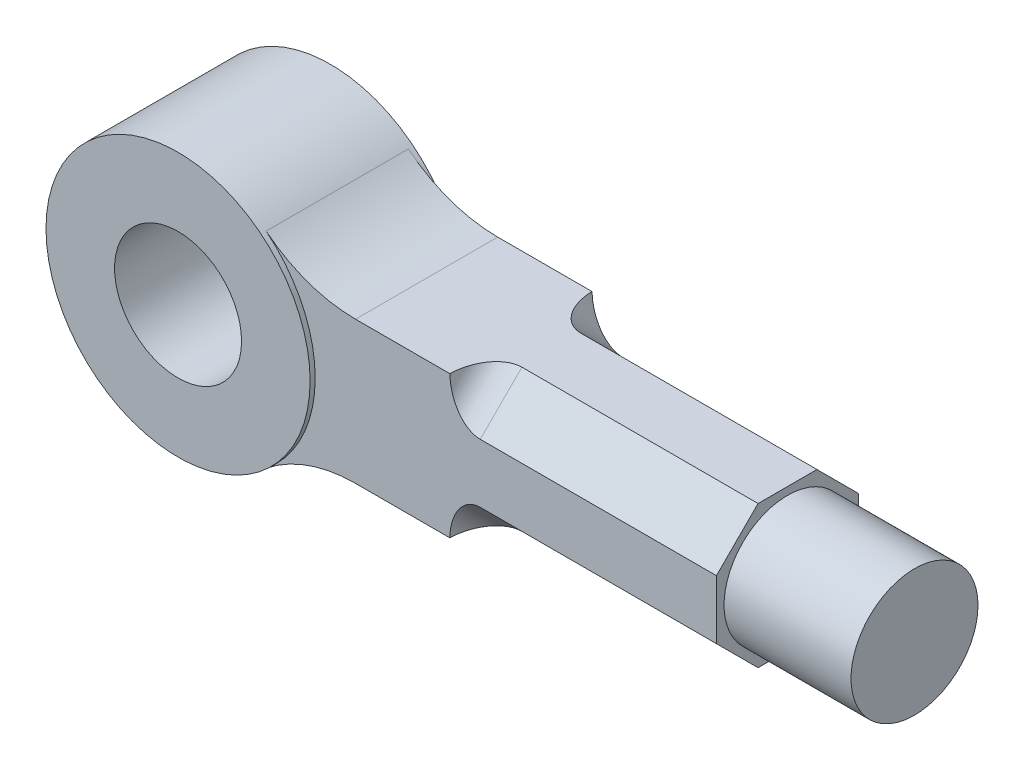
ISO-10303-21;
HEADER;
FILE_DESCRIPTION(('STEP AP214'),'2;1');
FILE_NAME('part.step','',(''),(''),'','','');
FILE_SCHEMA(('AUTOMOTIVE_DESIGN { 1 0 10303 214 1 1 1 1 }'));
ENDSEC;
DATA;
#1=APPLICATION_CONTEXT('core data for automotive mechanical design processes');
#2=APPLICATION_PROTOCOL_DEFINITION('international standard','automotive_design',2000,#1);
#3=PRODUCT_CONTEXT('',#1,'mechanical');
#4=PRODUCT('Part','Part','',(#3));
#5=PRODUCT_RELATED_PRODUCT_CATEGORY('part','',(#4));
#6=PRODUCT_DEFINITION_FORMATION('','',#4);
#7=PRODUCT_DEFINITION_CONTEXT('part definition',#1,'design');
#8=PRODUCT_DEFINITION('design','',#6,#7);
#9=PRODUCT_DEFINITION_SHAPE('','',#8);
#10=(LENGTH_UNIT() NAMED_UNIT(*) SI_UNIT(.MILLI.,.METRE.));
#11=(NAMED_UNIT(*) PLANE_ANGLE_UNIT() SI_UNIT($,.RADIAN.));
#12=(NAMED_UNIT(*) SI_UNIT($,.STERADIAN.) SOLID_ANGLE_UNIT());
#13=UNCERTAINTY_MEASURE_WITH_UNIT(LENGTH_MEASURE(1.E-05),#10,'distance_accuracy_value','');
#14=(GEOMETRIC_REPRESENTATION_CONTEXT(3) GLOBAL_UNCERTAINTY_ASSIGNED_CONTEXT((#13)) GLOBAL_UNIT_ASSIGNED_CONTEXT((#10,
#11,#12)) REPRESENTATION_CONTEXT('',''));
#15=CARTESIAN_POINT('',(0.,0.,0.));
#16=DIRECTION('',(0.,0.,1.));
#17=DIRECTION('',(1.,0.,0.));
#18=AXIS2_PLACEMENT_3D('',#15,#16,#17);
#19=CARTESIAN_POINT('',(0.,-14.,14.));
#20=DIRECTION('',(0.,-1.,0.));
#21=DIRECTION('',(0.,0.,-1.));
#22=AXIS2_PLACEMENT_3D('',#19,#20,#21);
#23=PLANE('',#22);
#24=DIRECTION('',(-1.,0.,0.));
#25=VECTOR('',#24,1.);
#26=CARTESIAN_POINT('',(0.,-14.,14.));
#27=LINE('',#26,#25);
#28=CARTESIAN_POINT('',(52.5033680345603,-14.,14.));
#29=VERTEX_POINT('',#28);
#30=CARTESIAN_POINT('',(33.9411254969543,-14.,14.));
#31=VERTEX_POINT('',#30);
#32=EDGE_CURVE('E255',#29,#31,#27,.T.);
#33=ORIENTED_EDGE('',*,*,#32,.T.);
#34=DIRECTION('',(0.,0.,-1.));
#35=VECTOR('',#34,1.);
#36=CARTESIAN_POINT('',(33.9411254969543,-14.,14.));
#37=LINE('',#36,#35);
#38=CARTESIAN_POINT('',(33.9411254969543,-14.,-14.));
#39=VERTEX_POINT('',#38);
#40=EDGE_CURVE('E221',#31,#39,#37,.T.);
#41=ORIENTED_EDGE('',*,*,#40,.T.);
#42=DIRECTION('',(-1.,0.,0.));
#43=VECTOR('',#42,1.);
#44=CARTESIAN_POINT('',(0.,-14.,-14.));
#45=LINE('',#44,#43);
#46=CARTESIAN_POINT('',(52.5033680345603,-14.,-14.));
#47=VERTEX_POINT('',#46);
#48=EDGE_CURVE('E263',#47,#39,#45,.T.);
#49=ORIENTED_EDGE('',*,*,#48,.F.);
#50=CARTESIAN_POINT('',(58.5,-14.,-14.2842712474619));
#51=DIRECTION('',(0.,-1.,0.));
#52=DIRECTION('',(0.,0.,1.));
#53=AXIS2_PLACEMENT_3D('',#50,#51,#52);
#54=ELLIPSE('',#53,8.48528137423857,6.);
#55=CARTESIAN_POINT('',(58.5,-14.,-5.79898987322333));
#56=VERTEX_POINT('',#55);
#57=EDGE_CURVE('E214',#47,#56,#54,.F.);
#58=ORIENTED_EDGE('',*,*,#57,.T.);
#59=DIRECTION('',(1.,0.,0.));
#60=VECTOR('',#59,1.);
#61=CARTESIAN_POINT('',(52.5,-14.,-5.79898987322333));
#62=LINE('',#61,#60);
#63=CARTESIAN_POINT('',(105.,-14.,-5.79898987322333));
#64=VERTEX_POINT('',#63);
#65=EDGE_CURVE('E166',#56,#64,#62,.T.);
#66=ORIENTED_EDGE('',*,*,#65,.T.);
#67=DIRECTION('',(0.,0.,-1.));
#68=VECTOR('',#67,1.);
#69=CARTESIAN_POINT('',(105.,-14.,14.));
#70=LINE('',#69,#68);
#71=CARTESIAN_POINT('',(105.,-14.,5.79898987322333));
#72=VERTEX_POINT('',#71);
#73=EDGE_CURVE('E173',#72,#64,#70,.T.);
#74=ORIENTED_EDGE('',*,*,#73,.F.);
#75=DIRECTION('',(1.,0.,0.));
#76=VECTOR('',#75,1.);
#77=CARTESIAN_POINT('',(52.5,-14.,5.79898987322333));
#78=LINE('',#77,#76);
#79=CARTESIAN_POINT('',(58.5,-14.,5.79898987322333));
#80=VERTEX_POINT('',#79);
#81=EDGE_CURVE('E283',#80,#72,#78,.T.);
#82=ORIENTED_EDGE('',*,*,#81,.F.);
#83=CARTESIAN_POINT('',(58.5,-14.,14.2842712474619));
#84=DIRECTION('',(0.,-1.,0.));
#85=DIRECTION('',(0.,0.,1.));
#86=AXIS2_PLACEMENT_3D('',#83,#84,#85);
#87=ELLIPSE('',#86,8.48528137423857,6.);
#88=EDGE_CURVE('E203',#80,#29,#87,.F.);
#89=ORIENTED_EDGE('',*,*,#88,.T.);
#90=EDGE_LOOP('',(#33,#41,#49,#58,#66,#74,#82,#89));
#91=FACE_BOUND('',#90,.T.);
#92=ADVANCED_FACE('F45',(#91),#23,.T.);
#93=CARTESIAN_POINT('',(105.,0.,14.));
#94=DIRECTION('',(1.,0.,0.));
#95=DIRECTION('',(0.,0.,-1.));
#96=AXIS2_PLACEMENT_3D('',#93,#94,#95);
#97=PLANE('',#96);
#98=CARTESIAN_POINT('',(105.,0.,0.));
#99=DIRECTION('',(1.,0.,0.));
#100=DIRECTION('',(0.,0.,-1.));
#101=AXIS2_PLACEMENT_3D('',#98,#99,#100);
#102=CIRCLE('',#101,12.5);
#103=CARTESIAN_POINT('',(105.,0.,-12.5));
#104=VERTEX_POINT('',#103);
#105=EDGE_CURVE('E12',#104,#104,#102,.T.);
#106=ORIENTED_EDGE('',*,*,#105,.F.);
#107=EDGE_LOOP('',(#106));
#108=FACE_BOUND('',#107,.T.);
#109=ORIENTED_EDGE('',*,*,#73,.T.);
#110=DIRECTION('',(0.,0.707106781186548,-0.707106781186548));
#111=VECTOR('',#110,1.);
#112=CARTESIAN_POINT('',(105.,-16.8994949366117,-2.89949493661166));
#113=LINE('',#112,#111);
#114=CARTESIAN_POINT('',(105.,-5.79898987322333,-14.));
#115=VERTEX_POINT('',#114);
#116=EDGE_CURVE('E170',#64,#115,#113,.T.);
#117=ORIENTED_EDGE('',*,*,#116,.T.);
#118=DIRECTION('',(0.,-1.,0.));
#119=VECTOR('',#118,1.);
#120=CARTESIAN_POINT('',(105.,0.,-14.));
#121=LINE('',#120,#119);
#122=CARTESIAN_POINT('',(105.,5.79898987322333,-14.));
#123=VERTEX_POINT('',#122);
#124=EDGE_CURVE('E168',#123,#115,#121,.T.);
#125=ORIENTED_EDGE('',*,*,#124,.F.);
#126=DIRECTION('',(0.,0.707106781186548,0.707106781186547));
#127=VECTOR('',#126,1.);
#128=CARTESIAN_POINT('',(105.,16.8994949366117,-2.89949493661167));
#129=LINE('',#128,#127);
#130=CARTESIAN_POINT('',(105.,14.,-5.79898987322334));
#131=VERTEX_POINT('',#130);
#132=EDGE_CURVE('E146',#123,#131,#129,.T.);
#133=ORIENTED_EDGE('',*,*,#132,.T.);
#134=DIRECTION('',(0.,0.,-1.));
#135=VECTOR('',#134,1.);
#136=CARTESIAN_POINT('',(105.,14.,14.));
#137=LINE('',#136,#135);
#138=CARTESIAN_POINT('',(105.,14.,5.79898987322333));
#139=VERTEX_POINT('',#138);
#140=EDGE_CURVE('E161',#139,#131,#137,.T.);
#141=ORIENTED_EDGE('',*,*,#140,.F.);
#142=DIRECTION('',(0.,-0.707106781186547,0.707106781186548));
#143=VECTOR('',#142,1.);
#144=CARTESIAN_POINT('',(105.,2.89949493661167,16.8994949366117));
#145=LINE('',#144,#143);
#146=CARTESIAN_POINT('',(105.,5.79898987322333,14.));
#147=VERTEX_POINT('',#146);
#148=EDGE_CURVE('E274',#139,#147,#145,.T.);
#149=ORIENTED_EDGE('',*,*,#148,.T.);
#150=DIRECTION('',(0.,-1.,0.));
#151=VECTOR('',#150,1.);
#152=CARTESIAN_POINT('',(105.,0.,14.));
#153=LINE('',#152,#151);
#154=CARTESIAN_POINT('',(105.,-5.79898987322333,14.));
#155=VERTEX_POINT('',#154);
#156=EDGE_CURVE('E178',#147,#155,#153,.T.);
#157=ORIENTED_EDGE('',*,*,#156,.T.);
#158=DIRECTION('',(0.,-0.707106781186547,-0.707106781186548));
#159=VECTOR('',#158,1.);
#160=CARTESIAN_POINT('',(105.,-2.89949493661167,16.8994949366117));
#161=LINE('',#160,#159);
#162=EDGE_CURVE('E260',#155,#72,#161,.T.);
#163=ORIENTED_EDGE('',*,*,#162,.T.);
#164=EDGE_LOOP('',(#109,#117,#125,#133,#141,#149,#157,#163));
#165=FACE_BOUND('',#164,.T.);
#166=ADVANCED_FACE('F163',(#108,#165),#97,.T.);
#167=CARTESIAN_POINT('',(0.,14.,14.));
#168=DIRECTION('',(0.,-1.,0.));
#169=DIRECTION('',(0.,0.,-1.));
#170=AXIS2_PLACEMENT_3D('',#167,#168,#169);
#171=PLANE('',#170);
#172=DIRECTION('',(-1.,0.,0.));
#173=VECTOR('',#172,1.);
#174=CARTESIAN_POINT('',(0.,14.,-14.));
#175=LINE('',#174,#173);
#176=CARTESIAN_POINT('',(52.5033680345603,14.,-14.));
#177=VERTEX_POINT('',#176);
#178=CARTESIAN_POINT('',(33.9411254969543,14.,-14.));
#179=VERTEX_POINT('',#178);
#180=EDGE_CURVE('E181',#177,#179,#175,.T.);
#181=ORIENTED_EDGE('',*,*,#180,.T.);
#182=DIRECTION('',(0.,0.,1.));
#183=VECTOR('',#182,1.);
#184=CARTESIAN_POINT('',(33.9411254969543,14.,14.));
#185=LINE('',#184,#183);
#186=CARTESIAN_POINT('',(33.9411254969543,14.,14.));
#187=VERTEX_POINT('',#186);
#188=EDGE_CURVE('E63',#179,#187,#185,.T.);
#189=ORIENTED_EDGE('',*,*,#188,.T.);
#190=DIRECTION('',(-1.,0.,0.));
#191=VECTOR('',#190,1.);
#192=CARTESIAN_POINT('',(0.,14.,14.));
#193=LINE('',#192,#191);
#194=CARTESIAN_POINT('',(52.5033680345603,14.,14.));
#195=VERTEX_POINT('',#194);
#196=EDGE_CURVE('E172',#195,#187,#193,.T.);
#197=ORIENTED_EDGE('',*,*,#196,.F.);
#198=CARTESIAN_POINT('',(58.5,14.,14.2842712474619));
#199=DIRECTION('',(0.,-1.,0.));
#200=DIRECTION('',(0.,0.,-1.));
#201=AXIS2_PLACEMENT_3D('',#198,#199,#200);
#202=ELLIPSE('',#201,8.48528137423857,6.);
#203=CARTESIAN_POINT('',(58.5,14.,5.79898987322333));
#204=VERTEX_POINT('',#203);
#205=EDGE_CURVE('E225',#195,#204,#202,.T.);
#206=ORIENTED_EDGE('',*,*,#205,.T.);
#207=DIRECTION('',(1.,0.,0.));
#208=VECTOR('',#207,1.);
#209=CARTESIAN_POINT('',(52.5,14.,5.79898987322333));
#210=LINE('',#209,#208);
#211=EDGE_CURVE('E154',#204,#139,#210,.T.);
#212=ORIENTED_EDGE('',*,*,#211,.T.);
#213=ORIENTED_EDGE('',*,*,#140,.T.);
#214=DIRECTION('',(1.,0.,0.));
#215=VECTOR('',#214,1.);
#216=CARTESIAN_POINT('',(52.5,14.,-5.79898987322334));
#217=LINE('',#216,#215);
#218=CARTESIAN_POINT('',(58.5,14.,-5.79898987322334));
#219=VERTEX_POINT('',#218);
#220=EDGE_CURVE('E143',#219,#131,#217,.T.);
#221=ORIENTED_EDGE('',*,*,#220,.F.);
#222=CARTESIAN_POINT('',(58.5,14.,-14.2842712474619));
#223=DIRECTION('',(0.,-1.,0.));
#224=DIRECTION('',(0.,0.,-1.));
#225=AXIS2_PLACEMENT_3D('',#222,#223,#224);
#226=ELLIPSE('',#225,8.48528137423857,6.);
#227=EDGE_CURVE('E213',#219,#177,#226,.T.);
#228=ORIENTED_EDGE('',*,*,#227,.T.);
#229=EDGE_LOOP('',(#181,#189,#197,#206,#212,#213,#221,#228));
#230=FACE_BOUND('',#229,.T.);
#231=ADVANCED_FACE('F167',(#230),#171,.F.);
#232=CARTESIAN_POINT('',(0.,0.,14.));
#233=DIRECTION('',(0.,0.,1.));
#234=DIRECTION('',(1.,0.,0.));
#235=AXIS2_PLACEMENT_3D('',#232,#233,#234);
#236=PLANE('',#235);
#237=DIRECTION('',(1.,0.,0.));
#238=VECTOR('',#237,1.);
#239=CARTESIAN_POINT('',(52.5,5.79898987322333,14.));
#240=LINE('',#239,#238);
#241=CARTESIAN_POINT('',(58.5,5.79898987322333,14.));
#242=VERTEX_POINT('',#241);
#243=EDGE_CURVE('E305',#242,#147,#240,.T.);
#244=ORIENTED_EDGE('',*,*,#243,.F.);
#245=CARTESIAN_POINT('',(58.5,14.2842712474619,14.));
#246=DIRECTION('',(0.,0.,1.));
#247=DIRECTION('',(0.,1.,0.));
#248=AXIS2_PLACEMENT_3D('',#245,#246,#247);
#249=ELLIPSE('',#248,8.48528137423857,6.);
#250=EDGE_CURVE('E217',#242,#195,#249,.F.);
#251=ORIENTED_EDGE('',*,*,#250,.T.);
#252=ORIENTED_EDGE('',*,*,#196,.T.);
#253=CARTESIAN_POINT('',(33.9411254969543,42.,14.));
#254=DIRECTION('',(0.,0.,1.));
#255=DIRECTION('',(1.,0.,0.));
#256=AXIS2_PLACEMENT_3D('',#253,#254,#255);
#257=CIRCLE('',#256,28.);
#258=CARTESIAN_POINT('',(16.3420233874224,20.2222222222222,14.));
#259=VERTEX_POINT('',#258);
#260=EDGE_CURVE('E46',#187,#259,#257,.F.);
#261=ORIENTED_EDGE('',*,*,#260,.T.);
#262=CARTESIAN_POINT('',(0.,0.,14.));
#263=DIRECTION('',(0.,0.,1.));
#264=DIRECTION('',(1.,0.,0.));
#265=AXIS2_PLACEMENT_3D('',#262,#263,#264);
#266=CIRCLE('',#265,26.);
#267=CARTESIAN_POINT('',(16.3420233874224,-20.2222222222222,14.));
#268=VERTEX_POINT('',#267);
#269=EDGE_CURVE('E242',#268,#259,#266,.T.);
#270=ORIENTED_EDGE('',*,*,#269,.F.);
#271=CARTESIAN_POINT('',(33.9411254969543,-42.,14.));
#272=DIRECTION('',(0.,0.,1.));
#273=DIRECTION('',(1.,0.,0.));
#274=AXIS2_PLACEMENT_3D('',#271,#272,#273);
#275=CIRCLE('',#274,28.);
#276=EDGE_CURVE('E240',#268,#31,#275,.F.);
#277=ORIENTED_EDGE('',*,*,#276,.T.);
#278=ORIENTED_EDGE('',*,*,#32,.F.);
#279=CARTESIAN_POINT('',(58.5,-14.2842712474619,14.));
#280=DIRECTION('',(0.,0.,1.));
#281=DIRECTION('',(0.,1.,0.));
#282=AXIS2_PLACEMENT_3D('',#279,#280,#281);
#283=ELLIPSE('',#282,8.48528137423857,6.);
#284=CARTESIAN_POINT('',(58.5,-5.79898987322333,14.));
#285=VERTEX_POINT('',#284);
#286=EDGE_CURVE('E206',#29,#285,#283,.F.);
#287=ORIENTED_EDGE('',*,*,#286,.T.);
#288=DIRECTION('',(1.,0.,0.));
#289=VECTOR('',#288,1.);
#290=CARTESIAN_POINT('',(52.5,-5.79898987322333,14.));
#291=LINE('',#290,#289);
#292=EDGE_CURVE('E301',#285,#155,#291,.T.);
#293=ORIENTED_EDGE('',*,*,#292,.T.);
#294=ORIENTED_EDGE('',*,*,#156,.F.);
#295=EDGE_LOOP('',(#244,#251,#252,#261,#270,#277,#278,#287,#293,#294));
#296=FACE_BOUND('',#295,.T.);
#297=ADVANCED_FACE('F243',(#296),#236,.T.);
#298=CARTESIAN_POINT('',(0.,0.,-14.));
#299=DIRECTION('',(0.,0.,1.));
#300=DIRECTION('',(1.,0.,0.));
#301=AXIS2_PLACEMENT_3D('',#298,#299,#300);
#302=PLANE('',#301);
#303=DIRECTION('',(1.,0.,0.));
#304=VECTOR('',#303,1.);
#305=CARTESIAN_POINT('',(52.5,-5.79898987322333,-14.));
#306=LINE('',#305,#304);
#307=CARTESIAN_POINT('',(58.5,-5.79898987322333,-14.));
#308=VERTEX_POINT('',#307);
#309=EDGE_CURVE('E270',#308,#115,#306,.T.);
#310=ORIENTED_EDGE('',*,*,#309,.F.);
#311=CARTESIAN_POINT('',(58.5,-14.2842712474619,-14.));
#312=DIRECTION('',(0.,0.,1.));
#313=DIRECTION('',(0.,-1.,0.));
#314=AXIS2_PLACEMENT_3D('',#311,#312,#313);
#315=ELLIPSE('',#314,8.48528137423857,6.);
#316=EDGE_CURVE('E208',#308,#47,#315,.T.);
#317=ORIENTED_EDGE('',*,*,#316,.T.);
#318=ORIENTED_EDGE('',*,*,#48,.T.);
#319=CARTESIAN_POINT('',(33.9411254969543,-42.,-14.));
#320=DIRECTION('',(0.,0.,1.));
#321=DIRECTION('',(1.,0.,0.));
#322=AXIS2_PLACEMENT_3D('',#319,#320,#321);
#323=CIRCLE('',#322,28.);
#324=CARTESIAN_POINT('',(16.3420233874224,-20.2222222222222,-14.));
#325=VERTEX_POINT('',#324);
#326=EDGE_CURVE('E234',#39,#325,#323,.T.);
#327=ORIENTED_EDGE('',*,*,#326,.T.);
#328=CARTESIAN_POINT('',(0.,0.,-14.));
#329=DIRECTION('',(0.,0.,1.));
#330=DIRECTION('',(1.,0.,0.));
#331=AXIS2_PLACEMENT_3D('',#328,#329,#330);
#332=CIRCLE('',#331,26.);
#333=CARTESIAN_POINT('',(16.3420233874224,20.2222222222222,-14.));
#334=VERTEX_POINT('',#333);
#335=EDGE_CURVE('E248',#325,#334,#332,.T.);
#336=ORIENTED_EDGE('',*,*,#335,.T.);
#337=CARTESIAN_POINT('',(33.9411254969543,42.,-14.));
#338=DIRECTION('',(0.,0.,1.));
#339=DIRECTION('',(1.,0.,0.));
#340=AXIS2_PLACEMENT_3D('',#337,#338,#339);
#341=CIRCLE('',#340,28.);
#342=EDGE_CURVE('E59',#334,#179,#341,.T.);
#343=ORIENTED_EDGE('',*,*,#342,.T.);
#344=ORIENTED_EDGE('',*,*,#180,.F.);
#345=CARTESIAN_POINT('',(58.5,14.2842712474619,-14.));
#346=DIRECTION('',(0.,0.,1.));
#347=DIRECTION('',(0.,-1.,0.));
#348=AXIS2_PLACEMENT_3D('',#345,#346,#347);
#349=ELLIPSE('',#348,8.48528137423857,6.);
#350=CARTESIAN_POINT('',(58.5,5.79898987322333,-14.));
#351=VERTEX_POINT('',#350);
#352=EDGE_CURVE('E220',#177,#351,#349,.T.);
#353=ORIENTED_EDGE('',*,*,#352,.T.);
#354=DIRECTION('',(1.,0.,0.));
#355=VECTOR('',#354,1.);
#356=CARTESIAN_POINT('',(52.5,5.79898987322333,-14.));
#357=LINE('',#356,#355);
#358=EDGE_CURVE('E157',#351,#123,#357,.T.);
#359=ORIENTED_EDGE('',*,*,#358,.T.);
#360=ORIENTED_EDGE('',*,*,#124,.T.);
#361=EDGE_LOOP('',(#310,#317,#318,#327,#336,#343,#344,#353,#359,#360));
#362=FACE_BOUND('',#361,.T.);
#363=ADVANCED_FACE('F267',(#362),#302,.F.);
#364=CARTESIAN_POINT('',(0.,0.,15.));
#365=DIRECTION('',(0.,0.,1.));
#366=DIRECTION('',(1.,0.,0.));
#367=AXIS2_PLACEMENT_3D('',#364,#365,#366);
#368=PLANE('',#367);
#369=CARTESIAN_POINT('',(0.,0.,15.));
#370=DIRECTION('',(0.,0.,1.));
#371=DIRECTION('',(1.,0.,0.));
#372=AXIS2_PLACEMENT_3D('',#369,#370,#371);
#373=CIRCLE('',#372,26.);
#374=CARTESIAN_POINT('',(26.,0.,15.));
#375=VERTEX_POINT('',#374);
#376=EDGE_CURVE('E188',#375,#375,#373,.T.);
#377=ORIENTED_EDGE('',*,*,#376,.T.);
#378=EDGE_LOOP('',(#377));
#379=FACE_BOUND('',#378,.T.);
#380=CARTESIAN_POINT('',(0.,0.,15.));
#381=DIRECTION('',(0.,0.,1.));
#382=DIRECTION('',(1.,0.,0.));
#383=AXIS2_PLACEMENT_3D('',#380,#381,#382);
#384=CIRCLE('',#383,12.5);
#385=CARTESIAN_POINT('',(12.5,0.,15.));
#386=VERTEX_POINT('',#385);
#387=EDGE_CURVE('E183',#386,#386,#384,.T.);
#388=ORIENTED_EDGE('',*,*,#387,.F.);
#389=EDGE_LOOP('',(#388));
#390=FACE_BOUND('',#389,.T.);
#391=ADVANCED_FACE('F334',(#379,#390),#368,.T.);
#392=CARTESIAN_POINT('',(0.,0.,-15.));
#393=DIRECTION('',(0.,0.,1.));
#394=DIRECTION('',(1.,0.,0.));
#395=AXIS2_PLACEMENT_3D('',#392,#393,#394);
#396=PLANE('',#395);
#397=CARTESIAN_POINT('',(0.,0.,-15.));
#398=DIRECTION('',(0.,0.,1.));
#399=DIRECTION('',(1.,0.,0.));
#400=AXIS2_PLACEMENT_3D('',#397,#398,#399);
#401=CIRCLE('',#400,26.);
#402=CARTESIAN_POINT('',(26.,0.,-15.));
#403=VERTEX_POINT('',#402);
#404=EDGE_CURVE('E190',#403,#403,#401,.T.);
#405=ORIENTED_EDGE('',*,*,#404,.F.);
#406=EDGE_LOOP('',(#405));
#407=FACE_BOUND('',#406,.T.);
#408=CARTESIAN_POINT('',(0.,0.,-15.));
#409=DIRECTION('',(0.,0.,1.));
#410=DIRECTION('',(1.,0.,0.));
#411=AXIS2_PLACEMENT_3D('',#408,#409,#410);
#412=CIRCLE('',#411,12.5);
#413=CARTESIAN_POINT('',(12.5,0.,-15.));
#414=VERTEX_POINT('',#413);
#415=EDGE_CURVE('E176',#414,#414,#412,.T.);
#416=ORIENTED_EDGE('',*,*,#415,.T.);
#417=EDGE_LOOP('',(#416));
#418=FACE_BOUND('',#417,.T.);
#419=ADVANCED_FACE('F337',(#407,#418),#396,.F.);
#420=CARTESIAN_POINT('',(0.,0.,15.));
#421=DIRECTION('',(0.,0.,-1.));
#422=DIRECTION('',(-1.,0.,0.));
#423=AXIS2_PLACEMENT_3D('',#420,#421,#422);
#424=CYLINDRICAL_SURFACE('',#423,26.);
#425=ORIENTED_EDGE('',*,*,#335,.F.);
#426=DIRECTION('',(0.,0.,-1.));
#427=VECTOR('',#426,1.);
#428=CARTESIAN_POINT('',(16.3420233874224,-20.2222222222222,15.));
#429=LINE('',#428,#427);
#430=EDGE_CURVE('E229',#325,#268,#429,.F.);
#431=ORIENTED_EDGE('',*,*,#430,.T.);
#432=ORIENTED_EDGE('',*,*,#269,.T.);
#433=DIRECTION('',(0.,0.,-1.));
#434=VECTOR('',#433,1.);
#435=CARTESIAN_POINT('',(16.3420233874224,20.2222222222222,15.));
#436=LINE('',#435,#434);
#437=EDGE_CURVE('E227',#259,#334,#436,.T.);
#438=ORIENTED_EDGE('',*,*,#437,.T.);
#439=EDGE_LOOP('',(#425,#431,#432,#438));
#440=FACE_BOUND('',#439,.T.);
#441=ORIENTED_EDGE('',*,*,#376,.F.);
#442=EDGE_LOOP('',(#441));
#443=FACE_BOUND('',#442,.T.);
#444=ORIENTED_EDGE('',*,*,#404,.T.);
#445=EDGE_LOOP('',(#444));
#446=FACE_BOUND('',#445,.T.);
#447=ADVANCED_FACE('F250',(#440,#443,#446),#424,.T.);
#448=CARTESIAN_POINT('',(0.,0.,15.));
#449=DIRECTION('',(0.,0.,-1.));
#450=DIRECTION('',(-1.,0.,0.));
#451=AXIS2_PLACEMENT_3D('',#448,#449,#450);
#452=CYLINDRICAL_SURFACE('',#451,12.5);
#453=ORIENTED_EDGE('',*,*,#387,.T.);
#454=EDGE_LOOP('',(#453));
#455=FACE_BOUND('',#454,.T.);
#456=ORIENTED_EDGE('',*,*,#415,.F.);
#457=EDGE_LOOP('',(#456));
#458=FACE_BOUND('',#457,.T.);
#459=ADVANCED_FACE('F327',(#455,#458),#452,.F.);
#460=CARTESIAN_POINT('',(52.5,5.79898987322333,-14.));
#461=DIRECTION('',(0.,0.707106781186547,-0.707106781186548));
#462=DIRECTION('',(0.,0.707106781186548,0.707106781186547));
#463=AXIS2_PLACEMENT_3D('',#460,#461,#462);
#464=PLANE('',#463);
#465=ORIENTED_EDGE('',*,*,#358,.F.);
#466=DIRECTION('',(0.,0.707106781186548,0.707106781186547));
#467=VECTOR('',#466,1.);
#468=CARTESIAN_POINT('',(58.5,14.,-5.79898987322333));
#469=LINE('',#468,#467);
#470=EDGE_CURVE('E155',#351,#219,#469,.T.);
#471=ORIENTED_EDGE('',*,*,#470,.T.);
#472=ORIENTED_EDGE('',*,*,#220,.T.);
#473=ORIENTED_EDGE('',*,*,#132,.F.);
#474=EDGE_LOOP('',(#465,#471,#472,#473));
#475=FACE_BOUND('',#474,.T.);
#476=ADVANCED_FACE('F149',(#475),#464,.T.);
#477=CARTESIAN_POINT('',(52.5,-14.,-5.79898987322333));
#478=DIRECTION('',(0.,-0.707106781186548,-0.707106781186548));
#479=DIRECTION('',(0.,0.707106781186548,-0.707106781186548));
#480=AXIS2_PLACEMENT_3D('',#477,#478,#479);
#481=PLANE('',#480);
#482=ORIENTED_EDGE('',*,*,#65,.F.);
#483=DIRECTION('',(0.,0.707106781186548,-0.707106781186548));
#484=VECTOR('',#483,1.);
#485=CARTESIAN_POINT('',(58.5,-5.79898987322333,-14.));
#486=LINE('',#485,#484);
#487=EDGE_CURVE('E198',#56,#308,#486,.T.);
#488=ORIENTED_EDGE('',*,*,#487,.T.);
#489=ORIENTED_EDGE('',*,*,#309,.T.);
#490=ORIENTED_EDGE('',*,*,#116,.F.);
#491=EDGE_LOOP('',(#482,#488,#489,#490));
#492=FACE_BOUND('',#491,.T.);
#493=ADVANCED_FACE('F288',(#492),#481,.T.);
#494=CARTESIAN_POINT('',(52.5,14.,5.79898987322333));
#495=DIRECTION('',(0.,0.707106781186548,0.707106781186547));
#496=DIRECTION('',(0.,-0.707106781186547,0.707106781186548));
#497=AXIS2_PLACEMENT_3D('',#494,#495,#496);
#498=PLANE('',#497);
#499=ORIENTED_EDGE('',*,*,#211,.F.);
#500=DIRECTION('',(0.,-0.707106781186547,0.707106781186548));
#501=VECTOR('',#500,1.);
#502=CARTESIAN_POINT('',(58.5,5.79898987322333,14.));
#503=LINE('',#502,#501);
#504=EDGE_CURVE('E205',#204,#242,#503,.T.);
#505=ORIENTED_EDGE('',*,*,#504,.T.);
#506=ORIENTED_EDGE('',*,*,#243,.T.);
#507=ORIENTED_EDGE('',*,*,#148,.F.);
#508=EDGE_LOOP('',(#499,#505,#506,#507));
#509=FACE_BOUND('',#508,.T.);
#510=ADVANCED_FACE('F381',(#509),#498,.T.);
#511=CARTESIAN_POINT('',(52.5,-5.79898987322333,14.));
#512=DIRECTION('',(0.,-0.707106781186548,0.707106781186547));
#513=DIRECTION('',(0.,-0.707106781186547,-0.707106781186548));
#514=AXIS2_PLACEMENT_3D('',#511,#512,#513);
#515=PLANE('',#514);
#516=ORIENTED_EDGE('',*,*,#292,.F.);
#517=DIRECTION('',(0.,-0.707106781186547,-0.707106781186548));
#518=VECTOR('',#517,1.);
#519=CARTESIAN_POINT('',(58.5,-14.,5.79898987322333));
#520=LINE('',#519,#518);
#521=EDGE_CURVE('E194',#285,#80,#520,.T.);
#522=ORIENTED_EDGE('',*,*,#521,.T.);
#523=ORIENTED_EDGE('',*,*,#81,.T.);
#524=ORIENTED_EDGE('',*,*,#162,.F.);
#525=EDGE_LOOP('',(#516,#522,#523,#524));
#526=FACE_BOUND('',#525,.T.);
#527=ADVANCED_FACE('F297',(#526),#515,.T.);
#528=CARTESIAN_POINT('',(58.5,-10.0416305603426,18.2426406871193));
#529=DIRECTION('',(0.,0.707106781186547,0.707106781186548));
#530=DIRECTION('',(0.,-0.707106781186548,0.707106781186547));
#531=AXIS2_PLACEMENT_3D('',#528,#529,#530);
#532=CYLINDRICAL_SURFACE('',#531,6.);
#533=ORIENTED_EDGE('',*,*,#521,.F.);
#534=ORIENTED_EDGE('',*,*,#286,.F.);
#535=ORIENTED_EDGE('',*,*,#88,.F.);
#536=EDGE_LOOP('',(#533,#534,#535));
#537=FACE_BOUND('',#536,.T.);
#538=ADVANCED_FACE('F299',(#537),#532,.F.);
#539=CARTESIAN_POINT('',(58.5,-18.2426406871193,-10.0416305603426));
#540=DIRECTION('',(0.,-0.707106781186548,0.707106781186548));
#541=DIRECTION('',(0.,-0.707106781186548,-0.707106781186548));
#542=AXIS2_PLACEMENT_3D('',#539,#540,#541);
#543=CYLINDRICAL_SURFACE('',#542,6.);
#544=ORIENTED_EDGE('',*,*,#57,.F.);
#545=ORIENTED_EDGE('',*,*,#316,.F.);
#546=ORIENTED_EDGE('',*,*,#487,.F.);
#547=EDGE_LOOP('',(#544,#545,#546));
#548=FACE_BOUND('',#547,.T.);
#549=ADVANCED_FACE('F292',(#548),#543,.F.);
#550=CARTESIAN_POINT('',(58.5,10.0416305603426,-18.2426406871193));
#551=DIRECTION('',(0.,-0.707106781186548,-0.707106781186547));
#552=DIRECTION('',(0.,0.707106781186547,-0.707106781186548));
#553=AXIS2_PLACEMENT_3D('',#550,#551,#552);
#554=CYLINDRICAL_SURFACE('',#553,6.);
#555=ORIENTED_EDGE('',*,*,#352,.F.);
#556=ORIENTED_EDGE('',*,*,#227,.F.);
#557=ORIENTED_EDGE('',*,*,#470,.F.);
#558=EDGE_LOOP('',(#555,#556,#557));
#559=FACE_BOUND('',#558,.T.);
#560=ADVANCED_FACE('F350',(#559),#554,.F.);
#561=CARTESIAN_POINT('',(58.5,18.2426406871193,10.0416305603426));
#562=DIRECTION('',(0.,0.707106781186547,-0.707106781186548));
#563=DIRECTION('',(0.,0.707106781186548,0.707106781186547));
#564=AXIS2_PLACEMENT_3D('',#561,#562,#563);
#565=CYLINDRICAL_SURFACE('',#564,6.);
#566=ORIENTED_EDGE('',*,*,#504,.F.);
#567=ORIENTED_EDGE('',*,*,#205,.F.);
#568=ORIENTED_EDGE('',*,*,#250,.F.);
#569=EDGE_LOOP('',(#566,#567,#568));
#570=FACE_BOUND('',#569,.T.);
#571=ADVANCED_FACE('F349',(#570),#565,.F.);
#572=CARTESIAN_POINT('',(33.9411254969543,-42.,15.));
#573=DIRECTION('',(0.,0.,-1.));
#574=DIRECTION('',(-1.,0.,0.));
#575=AXIS2_PLACEMENT_3D('',#572,#573,#574);
#576=CYLINDRICAL_SURFACE('',#575,28.);
#577=ORIENTED_EDGE('',*,*,#276,.F.);
#578=ORIENTED_EDGE('',*,*,#430,.F.);
#579=ORIENTED_EDGE('',*,*,#326,.F.);
#580=ORIENTED_EDGE('',*,*,#40,.F.);
#581=EDGE_LOOP('',(#577,#578,#579,#580));
#582=FACE_BOUND('',#581,.T.);
#583=ADVANCED_FACE('F294',(#582),#576,.F.);
#584=CARTESIAN_POINT('',(33.9411254969543,42.,15.));
#585=DIRECTION('',(0.,0.,-1.));
#586=DIRECTION('',(-1.,0.,0.));
#587=AXIS2_PLACEMENT_3D('',#584,#585,#586);
#588=CYLINDRICAL_SURFACE('',#587,28.);
#589=ORIENTED_EDGE('',*,*,#260,.F.);
#590=ORIENTED_EDGE('',*,*,#188,.F.);
#591=ORIENTED_EDGE('',*,*,#342,.F.);
#592=ORIENTED_EDGE('',*,*,#437,.F.);
#593=EDGE_LOOP('',(#589,#590,#591,#592));
#594=FACE_BOUND('',#593,.T.);
#595=ADVANCED_FACE('F42',(#594),#588,.F.);
#596=CARTESIAN_POINT('',(130.,0.,0.));
#597=DIRECTION('',(-1.,0.,0.));
#598=DIRECTION('',(0.,0.,1.));
#599=AXIS2_PLACEMENT_3D('',#596,#597,#598);
#600=CYLINDRICAL_SURFACE('',#599,12.5);
#601=CARTESIAN_POINT('',(130.,0.,0.));
#602=DIRECTION('',(1.,0.,0.));
#603=DIRECTION('',(0.,0.,-1.));
#604=AXIS2_PLACEMENT_3D('',#601,#602,#603);
#605=CIRCLE('',#604,12.5);
#606=CARTESIAN_POINT('',(130.,0.,-12.5));
#607=VERTEX_POINT('',#606);
#608=EDGE_CURVE('E268',#607,#607,#605,.T.);
#609=ORIENTED_EDGE('',*,*,#608,.F.);
#610=EDGE_LOOP('',(#609));
#611=FACE_BOUND('',#610,.T.);
#612=ORIENTED_EDGE('',*,*,#105,.T.);
#613=EDGE_LOOP('',(#612));
#614=FACE_BOUND('',#613,.T.);
#615=ADVANCED_FACE('F315',(#611,#614),#600,.T.);
#616=CARTESIAN_POINT('',(130.,0.,0.));
#617=DIRECTION('',(1.,0.,0.));
#618=DIRECTION('',(0.,0.,-1.));
#619=AXIS2_PLACEMENT_3D('',#616,#617,#618);
#620=PLANE('',#619);
#621=ORIENTED_EDGE('',*,*,#608,.T.);
#622=EDGE_LOOP('',(#621));
#623=FACE_BOUND('',#622,.T.);
#624=ADVANCED_FACE('F309',(#623),#620,.T.);
#625=CLOSED_SHELL('',(#92,#166,#231,#297,#363,#391,#419,#447,#459,#476,#493,#510,#527,#538,#549,
#560,#571,#583,#595,#615,#624));
#626=MANIFOLD_SOLID_BREP('B2',#625);
#627=ADVANCED_BREP_SHAPE_REPRESENTATION('',(#18,#626),#14);
#628=SHAPE_DEFINITION_REPRESENTATION(#9,#627);
ENDSEC;
END-ISO-10303-21;
